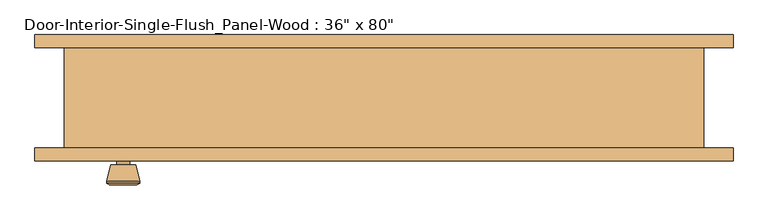
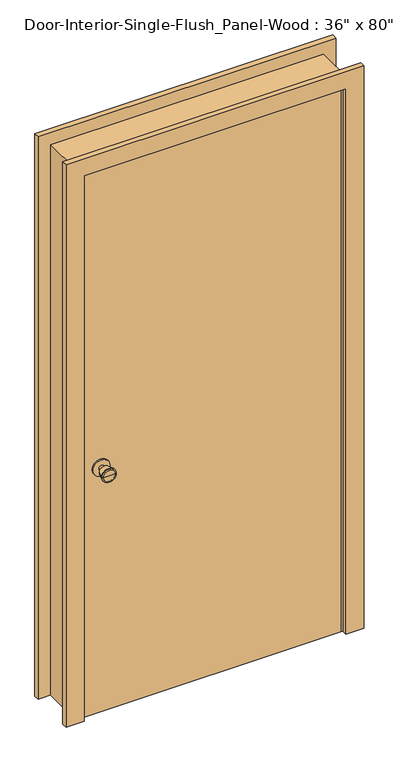
"""IFC4 building model written with IfcOpenShell, lengths in millimetres: door geometry."""

from ifc_helpers import new_model, si_unit, point, frame, frame_2d, origin, origin_with_axes, place, context, project, spatial, polyline, circle_curve, trimmed, segment, composite_curve, outline, extrude, faceted_brep, source, transform, mapped, element, save
from ifc_brep_helpers import plane_surface, cylinder_surface, revolved_surface, advanced_brep


def door_acdcadbb(model_context):
    return source(origin(), model_context, "Body", "SolidModel", [
        advanced_brep(
        [(-393.7, -32.1, 914.4), (-403.7, -32.1, 914.4), (-383.7, -32.1, 914.4), (-373.2241324, 16.9, 914.4), (-414.1758676, 16.9, 914.4), (-393.7, 16.9, 914.4), (-368.7, 15.0721319, 914.4), (-418.7, 15.0721319, 914.4), (-368.7, 11.6084537, 914.4), (-418.7, 11.6084537, 914.4), (-375.063764, -13.1, 914.4), (-412.336236, -13.1, 914.4), (-383.7, -13.1, 914.4), (-403.7, -13.1, 914.4)],
        [
            (0, 1),
            (1, 2, circle_curve(frame((-393.7, -32.1, 914.4), z_axis=(0.0, -1.0, 0.0), x_axis=(-1.0, 0.0, 0.0)), 10.0)),
            (2, 0),
            (2, 1, circle_curve(frame((-393.7, -32.1, 914.4), z_axis=(0.0, -1.0, 0.0), x_axis=(-1.0, 0.0, 0.0)), 10.0)),
            (3, 4, circle_curve(frame((-393.7, 16.9, 914.4), z_axis=(0.0, 1.0, 0.0), x_axis=(-1.0, 0.0, 0.0)), 20.4758676)),
            (4, 5),
            (5, 3),
            (4, 3, circle_curve(frame((-393.7, 16.9, 914.4), z_axis=(0.0, 1.0, 0.0), x_axis=(-1.0, 0.0, 0.0)), 20.4758676)),
            (6, 7, circle_curve(frame((-393.7, 15.0721319, 914.4), z_axis=(0.0, 1.0, 0.0), x_axis=(-1.0, 0.0, 0.0)), 25.0)),
            (7, 4),
            (3, 6),
            (7, 6, circle_curve(frame((-393.7, 15.0721319, 914.4), z_axis=(0.0, 1.0, 0.0), x_axis=(-1.0, 0.0, 0.0)), 25.0)),
            (8, 9, circle_curve(frame((-393.7, 11.6084537, 914.4), z_axis=(0.0, 1.0, 0.0), x_axis=(-1.0, 0.0, 0.0)), 25.0)),
            (9, 7),
            (6, 8),
            (9, 8, circle_curve(frame((-393.7, 11.6084537, 914.4), z_axis=(0.0, 1.0, 0.0), x_axis=(-1.0, 0.0, 0.0)), 25.0)),
            (10, 11, circle_curve(frame((-393.7, -13.1, 914.4), z_axis=(0.0, 1.0, 0.0), x_axis=(-1.0, 0.0, 0.0)), 18.636236)),
            (11, 9),
            (8, 10),
            (11, 10, circle_curve(frame((-393.7, -13.1, 914.4), z_axis=(0.0, 1.0, 0.0), x_axis=(-1.0, 0.0, 0.0)), 18.636236)),
            (12, 13, circle_curve(frame((-393.7, -13.1, 914.4), z_axis=(0.0, 1.0, 0.0), x_axis=(-1.0, 0.0, 0.0)), 10.0)),
            (13, 11),
            (10, 12),
            (13, 12, circle_curve(frame((-393.7, -13.1, 914.4), z_axis=(0.0, 1.0, 0.0), x_axis=(-1.0, 0.0, 0.0)), 10.0)),
            (1, 13),
            (12, 2),
        ],
        [
            plane_surface(frame((-393.7, -32.1, 914.4), z_axis=(0.0, -1.0, 0.0), x_axis=(-1.0, 0.0, 0.0))),
            plane_surface(frame((-393.7, 16.9, 914.4), z_axis=(0.0, 1.0, 0.0), x_axis=(-1.0, 0.0, 0.0))),
            revolved_surface(polyline([(-414.1758676, 16.9, 914.4), (-418.7, 15.0721319, 914.4)]), (-393.7, -32.1, 914.4), (0.0, -1.0, 0.0)),
            cylinder_surface(frame((-393.7, -32.1, 914.4), z_axis=(0.0, -1.0, 0.0), x_axis=(-1.0, 0.0, 0.0)), 25.0),
            revolved_surface(polyline([(-418.7, 11.6084537, 914.4), (-412.336236, -13.1, 914.4)]), (-393.7, -32.1, 914.4), (0.0, -1.0, 0.0)),
            plane_surface(frame((-393.7, -13.1, 914.4), z_axis=(0.0, -1.0, 0.0), x_axis=(-1.0, 0.0, 0.0))),
            cylinder_surface(frame((-393.7, -32.1, 914.4), z_axis=(0.0, -1.0, 0.0), x_axis=(-1.0, 0.0, 0.0)), 10.0),
        ],
        [
            (0, [[1, 2, 3]]),
            (0, [[-3, 4, -1]]),
            (1, [[5, 6, 7]]),
            (1, [[8, -7, -6]]),
            (2, [[9, 10, -5, 11]]),
            (2, [[12, -11, -8, -10]]),
            (3, [[13, 14, -9, 15]]),
            (3, [[16, -15, -12, -14]]),
            (4, [[17, 18, -13, 19]]),
            (4, [[20, -19, -16, -18]]),
            (5, [[21, 22, -17, 23]]),
            (5, [[24, -23, -20, -22]]),
            (6, [[-2, 25, -21, 26]]),
            (6, [[-4, -26, -24, -25]]),
        ],
    ),
        extrude(outline(composite_curve([segment(trimmed(circle_curve(frame_2d((914.4, -393.7)), 30.0), [point((914.4, -423.7))], [point((914.4, -363.7))], False, "CARTESIAN"), True, "CONTINUOUS"), segment(trimmed(circle_curve(frame_2d((914.4, -393.7)), 30.0), [point((914.4, -363.7))], [point((914.4, -423.7))], False, "CARTESIAN"), True, "CONTINUOUS")], self_intersect=False)), frame((0.0, -38.1, 0.0), z_axis=(0.0, 1.0, 0.0), x_axis=(0.0, 0.0, 1.0)), (0.0, 0.0, 1.0), 6.0),
        advanced_brep(
        [(-393.7, -79.025, 914.4), (-383.7, -79.025, 914.4), (-403.7, -79.025, 914.4), (-373.2241324, -128.025, 914.4), (-393.7, -128.025, 914.4), (-414.1758676, -128.025, 914.4), (-368.7, -126.1971319, 914.4), (-418.7, -126.1971319, 914.4), (-368.7, -122.7334537, 914.4), (-418.7, -122.7334537, 914.4), (-375.063764, -98.025, 914.4), (-412.336236, -98.025, 914.4), (-383.7, -98.025, 914.4), (-403.7, -98.025, 914.4)],
        [
            (0, 1),
            (1, 2, circle_curve(frame((-393.7, -79.025, 914.4), z_axis=(0.0, 1.0, 0.0), x_axis=(-1.0, 0.0, 0.0)), 10.0)),
            (2, 0),
            (2, 1, circle_curve(frame((-393.7, -79.025, 914.4), z_axis=(0.0, 1.0, 0.0), x_axis=(-1.0, 0.0, 0.0)), 10.0)),
            (3, 4),
            (4, 5),
            (5, 3, circle_curve(frame((-393.7, -128.025, 914.4), z_axis=(0.0, -1.0, 0.0), x_axis=(-1.0, 0.0, 0.0)), 20.4758676)),
            (3, 5, circle_curve(frame((-393.7, -128.025, 914.4), z_axis=(0.0, -1.0, 0.0), x_axis=(-1.0, 0.0, 0.0)), 20.4758676)),
            (6, 3),
            (5, 7),
            (7, 6, circle_curve(frame((-393.7, -126.1971319, 914.4), z_axis=(0.0, -1.0, 0.0), x_axis=(-1.0, 0.0, 0.0)), 25.0)),
            (6, 7, circle_curve(frame((-393.7, -126.1971319, 914.4), z_axis=(0.0, -1.0, 0.0), x_axis=(-1.0, 0.0, 0.0)), 25.0)),
            (8, 6),
            (7, 9),
            (9, 8, circle_curve(frame((-393.7, -122.7334537, 914.4), z_axis=(0.0, -1.0, 0.0), x_axis=(-1.0, 0.0, 0.0)), 25.0)),
            (8, 9, circle_curve(frame((-393.7, -122.7334537, 914.4), z_axis=(0.0, -1.0, 0.0), x_axis=(-1.0, 0.0, 0.0)), 25.0)),
            (10, 8),
            (9, 11),
            (11, 10, circle_curve(frame((-393.7, -98.025, 914.4), z_axis=(0.0, -1.0, 0.0), x_axis=(-1.0, 0.0, 0.0)), 18.636236)),
            (10, 11, circle_curve(frame((-393.7, -98.025, 914.4), z_axis=(0.0, -1.0, 0.0), x_axis=(-1.0, 0.0, 0.0)), 18.636236)),
            (12, 10),
            (11, 13),
            (13, 12, circle_curve(frame((-393.7, -98.025, 914.4), z_axis=(0.0, -1.0, 0.0), x_axis=(-1.0, 0.0, 0.0)), 10.0)),
            (12, 13, circle_curve(frame((-393.7, -98.025, 914.4), z_axis=(0.0, -1.0, 0.0), x_axis=(-1.0, 0.0, 0.0)), 10.0)),
            (1, 12),
            (13, 2),
        ],
        [
            plane_surface(frame((-393.7, -79.025, 914.4), z_axis=(0.0, 1.0, 0.0), x_axis=(-1.0, 0.0, 0.0))),
            plane_surface(frame((-393.7, -128.025, 914.4), z_axis=(0.0, -1.0, 0.0), x_axis=(-1.0, 0.0, 0.0))),
            revolved_surface(polyline([(-414.1758676, -128.025, 914.4), (-418.7, -126.1971319, 914.4)]), (-393.7, -79.025, 914.4), (0.0, 1.0, 0.0)),
            cylinder_surface(frame((-393.7, -79.025, 914.4), z_axis=(0.0, 1.0, 0.0), x_axis=(-1.0, 0.0, 0.0)), 25.0),
            revolved_surface(polyline([(-418.7, -122.7334537, 914.4), (-412.336236, -98.025, 914.4)]), (-393.7, -79.025, 914.4), (0.0, 1.0, 0.0)),
            plane_surface(frame((-393.7, -98.025, 914.4), z_axis=(0.0, 1.0, 0.0), x_axis=(-1.0, 0.0, 0.0))),
            cylinder_surface(frame((-393.7, -79.025, 914.4), z_axis=(0.0, 1.0, 0.0), x_axis=(-1.0, 0.0, 0.0)), 10.0),
        ],
        [
            (0, [[1, 2, 3]]),
            (0, [[-3, 4, -1]]),
            (1, [[5, 6, 7]]),
            (1, [[-6, -5, 8]]),
            (2, [[9, -7, 10, 11]]),
            (2, [[-10, -8, -9, 12]]),
            (3, [[13, -11, 14, 15]]),
            (3, [[-14, -12, -13, 16]]),
            (4, [[17, -15, 18, 19]]),
            (4, [[-18, -16, -17, 20]]),
            (5, [[21, -19, 22, 23]]),
            (5, [[-22, -20, -21, 24]]),
            (6, [[25, -23, 26, -2]]),
            (6, [[-26, -24, -25, -4]]),
        ],
    ),
        extrude(outline(composite_curve([segment(trimmed(circle_curve(frame_2d((914.4, -393.7)), 30.0), [point((914.4, -423.7))], [point((914.4, -363.7))], False, "CARTESIAN"), True, "CONTINUOUS"), segment(trimmed(circle_curve(frame_2d((914.4, -393.7)), 30.0), [point((914.4, -363.7))], [point((914.4, -423.7))], False, "CARTESIAN"), True, "CONTINUOUS")], self_intersect=False)), frame((0.0, -79.025, 0.0), z_axis=(0.0, 1.0, 0.0), x_axis=(0.0, 0.0, 1.0)), (0.0, 0.0, 1.0), 6.0),
        extrude(outline(polyline([(457.2, -38.1), (457.2, -73.025), (-457.2, -73.025), (-457.2, -38.1), (457.2, -38.1)])), origin_with_axes(), (0.0, 0.0, 1.0), 2032.0),
        faceted_brep([(482.6, -73.025, 0.0), (457.2, -73.025, 0.0), (457.2, -38.1, 0.0), (444.5, -38.1, 0.0), (444.5, -3.175, 0.0), (457.2, -3.175, 0.0), (457.2, 79.375, 0.0), (482.6, 79.375, 0.0), (482.6, 79.375, 2057.4), (482.6, -73.025, 2057.4), (457.2, 79.375, 2032.0), (-457.2, 79.375, 2032.0), (-457.2, 79.375, 0.0), (-482.6, 79.375, 0.0), (-482.6, 79.375, 2057.4), (457.2, -3.175, 2032.0), (444.5, -3.175, 2019.3), (-444.5, -3.175, 2019.3), (-444.5, -3.175, 0.0), (-457.2, -3.175, 0.0), (-457.2, -3.175, 2032.0), (444.5, -38.1, 2019.3), (457.2, -38.1, 2032.0), (-457.2, -38.1, 2032.0), (-457.2, -38.1, 0.0), (-444.5, -38.1, 0.0), (-444.5, -38.1, 2019.3), (457.2, -73.025, 2032.0), (-482.6, -73.025, 2057.4), (-482.6, -73.025, 0.0), (-457.2, -73.025, 0.0), (-457.2, -73.025, 2032.0)], [[[0, 1, 2, 3, 4, 5, 6, 7]], [[7, 8, 9, 0]], [[6, 10, 11, 12, 13, 14, 8, 7]], [[5, 15, 10, 6]], [[4, 16, 17, 18, 19, 20, 15, 5]], [[3, 21, 16, 4]], [[2, 22, 23, 24, 25, 26, 21, 3]], [[1, 27, 22, 2]], [[0, 9, 28, 29, 30, 31, 27, 1]], [[8, 14, 28, 9]], [[15, 20, 11, 10]], [[21, 26, 17, 16]], [[27, 31, 23, 22]], [[29, 13, 12, 19, 18, 25, 24, 30]], [[14, 13, 29, 28]], [[20, 19, 12, 11]], [[26, 25, 18, 17]], [[31, 30, 24, 23]]]),
        extrude(outline(polyline([(0.0, 527.05), (2101.85, 527.05), (2101.85, -527.05), (0.0, -527.05), (0.0, -463.55), (2038.35, -463.55), (2038.35, 463.55), (0.0, 463.55), (0.0, 527.05)])), frame((0.0, 79.375, 0.0), z_axis=(0.0, 1.0, 0.0), x_axis=(0.0, 0.0, 1.0)), (0.0, 0.0, 1.0), 19.05),
        extrude(outline(polyline([(0.0, 527.05), (2101.85, 527.05), (2101.85, -527.05), (0.0, -527.05), (0.0, -463.55), (2038.35, -463.55), (2038.35, 463.55), (0.0, 463.55), (0.0, 527.05)])), frame((0.0, -92.075, 0.0), z_axis=(0.0, 1.0, 0.0), x_axis=(0.0, 0.0, 1.0)), (0.0, 0.0, 1.0), 19.05),
    ])


if __name__ == "__main__":
    model = new_model("IFC4")
    model_context = context("Model", 3, world=origin())
    ifc_project = project(units=[si_unit("LENGTHUNIT", "METRE", prefix="MILLI")], contexts=[model_context])
    site = spatial("IfcSite", under=ifc_project)
    building = spatial("IfcBuilding", under=site)
    placement = place(None, origin())
    door_shape = door_acdcadbb(model_context)
    element("IfcDoor", 1, ObjectType="Door-Interior-Single-Flush_Panel-Wood : 36\" x 80\"", at=placement, inside=building, context=model_context, shape_type="MappedRepresentation", body=[
        mapped(door_shape, transform((0.0, 0.0, 0.0), x_axis=(1.0, 0.0, 0.0), y_axis=(0.0, 1.0, 0.0), z_axis=(0.0, 0.0, 1.0))),
    ])
    save(model, "model.ifc")

# Revit data of these elements
# Type "Door-Interior-Single-Flush_Panel-Wood : 36\" x 80\""
#   Type Mark = "9"
#   Assembly Code = "C1020300"
#   Analytic Construction = "Wooden"
#   Thickness = 0' - 1 3/8"
#   Thermal Resistance (R) = 2.5876 (h·ft²·°F)/BTU
#   Swing Angle [instance default] = 90.00°
#   Rough Width = 3' - 2"
#   Rough Height = 6' - 9"
#   Height = 6' - 8"
#   Width = 3' - 0"
#   Heat Transfer Coefficient (U) = 0.3865 BTU/(h·ft²·°F)
#   Trim Material = Cherry
#   Panel Material = Cherry
#   Frame Material = Cherry
#   Door Handle Material = Aluminum
#   Visual Light Transmittance = 0
#   Solar Heat Gain Coefficient = 0
#   Wall Closure = (empty or 0)
#   Function = (empty or 0)
# Element 1 (IfcDoor, "Door-Interior-Single-Flush_Panel-Wood : 36\" x 80\"")
#   Materials on its faces: "Cherry", "Aluminum"
# Materials
#   "Cherry": class "Wood", colour RGB 226 177 128, transparency 0, Description = "Prunus Serotina", Cost = 0
#   "Aluminum": class "Metal", colour RGB 247 247 247, transparency 0, Description = "Aluminum 6061", Cost = 0
